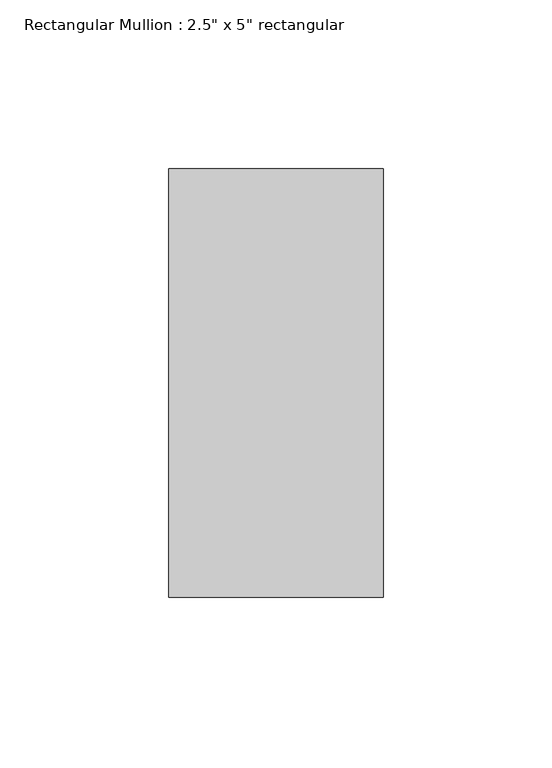
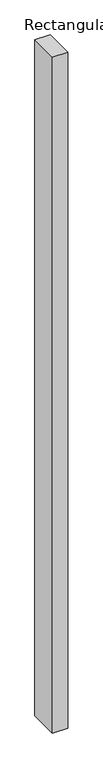
"""IFC4 building model written with IfcOpenShell, lengths in millimetres: member geometry."""

from ifc_helpers import new_model, si_unit, frame, origin, place, context, project, spatial, polyline, outline, extrude, source, transform, mapped, element, save


def member_8cef0660(model_context):
    return source(origin(), model_context, "Body", "SweptSolid", [
        extrude(outline(polyline([(31.75, 63.5), (31.75, -63.5), (-31.75, -63.5), (-31.75, 63.5), (31.75, 63.5)])), frame((0.0, 0.0, -2984.5), z_axis=(0.0, 0.0, 1.0), x_axis=(1.0, 0.0, 0.0)), (0.0, 0.0, 1.0), 2984.5),
    ])


if __name__ == "__main__":
    model = new_model("IFC4")
    model_context = context("Model", 3, world=origin())
    ifc_project = project(units=[si_unit("LENGTHUNIT", "METRE", prefix="MILLI")], contexts=[model_context])
    site = spatial("IfcSite", under=ifc_project)
    building = spatial("IfcBuilding", under=site)
    placement = place(None, origin())
    member_shape = member_8cef0660(model_context)
    element("IfcMember", 1, ObjectType="Rectangular Mullion : 2.5\" x 5\" rectangular", at=placement, inside=building, context=model_context, shape_type="MappedRepresentation", body=[
        mapped(member_shape, transform((0.0, 0.0, 0.0), x_axis=(1.0, 0.0, 0.0), y_axis=(0.0, 1.0, 0.0), z_axis=(0.0, 0.0, 1.0))),
    ])
    save(model, "model.ifc")

# Revit data of these elements
# Type "Rectangular Mullion : 2.5\" x 5\" rectangular"
#   built-in parameter 1007304 = 0.416667 (stored number, unit not read)
#   built-in parameter 1007301 = 0.104167 (stored number, unit not read)
#   built-in parameter 1007300 = 0.104167 (stored number, unit not read)
# Element 1 (IfcMember, "Rectangular Mullion : 2.5\" x 5\" rectangular")
#   Materials on its faces: "Aluminum"
# Materials
#   "Aluminum": class "Metal", colour RGB 247 247 247, transparency 0, Description = "Aluminum 6061", Cost = 0
